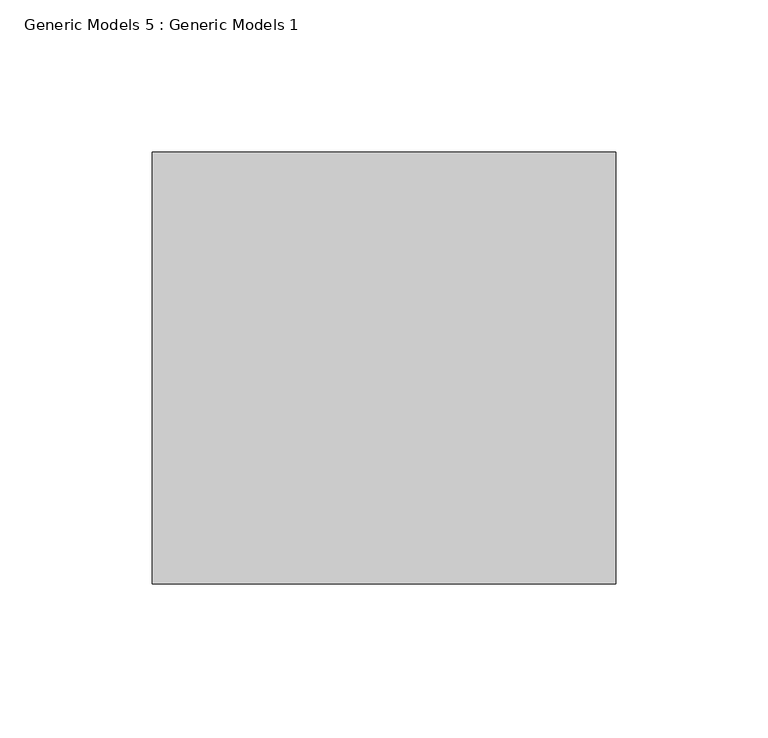
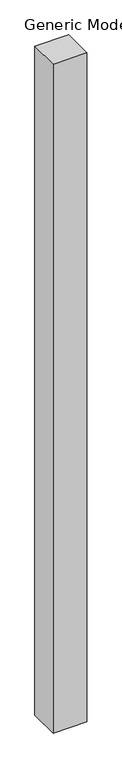
"""IFC4 building model written with IfcOpenShell, lengths in millimetres: proxy geometry, Generic Models 5 : Generic Models 1."""

from ifc_helpers import new_model, si_unit, origin, origin_with_axes, place, context, project, spatial, polyline, outline, extrude, source, transform, mapped, element, save


def generic_models_5_generic_models_1_4439abc4(model_context):
    return source(origin(), model_context, "Body", "SweptSolid", [
        extrude(outline(polyline([(-10727.8168582, -5471.7273102), (-10575.4168582, -5471.7273102), (-10575.4168582, -5613.7098142), (-10727.8168582, -5613.7098142), (-10727.8168582, -5471.7273102)])), origin_with_axes(), (0.0, 0.0, 1.0), 3200.4),
    ])


if __name__ == "__main__":
    model = new_model("IFC4")
    model_context = context("Model", 3, world=origin())
    ifc_project = project(units=[si_unit("LENGTHUNIT", "METRE", prefix="MILLI")], contexts=[model_context])
    site = spatial("IfcSite", under=ifc_project)
    building = spatial("IfcBuilding", under=site)
    placement = place(None, origin())
    generic_models_5_generic_models_1_shape = generic_models_5_generic_models_1_4439abc4(model_context)
    element("IfcBuildingElementProxy", 1, Name="Generic Models 5 : Generic Models 1", ObjectType="Generic Models 5 : Generic Models 1", at=placement, inside=building, context=model_context, shape_type="MappedRepresentation", body=[
        mapped(generic_models_5_generic_models_1_shape, transform((0.0, 0.0, 0.0), x_axis=(1.0, 0.0, 0.0), y_axis=(0.0, 1.0, 0.0), z_axis=(0.0, 0.0, 1.0))),
    ])
    save(model, "model.ifc")
